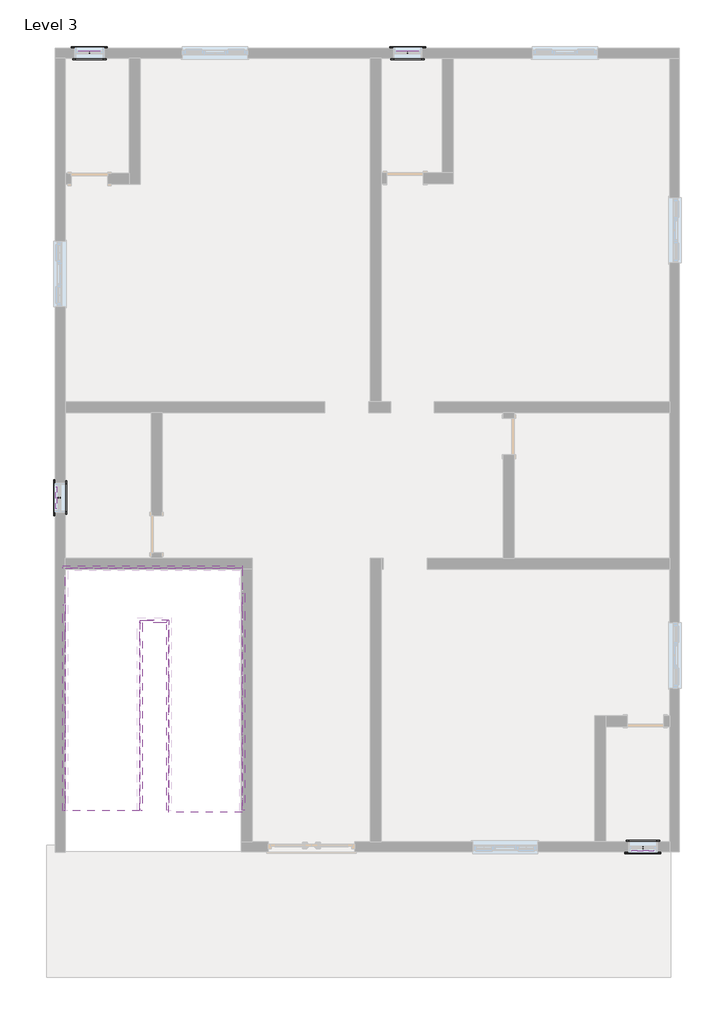
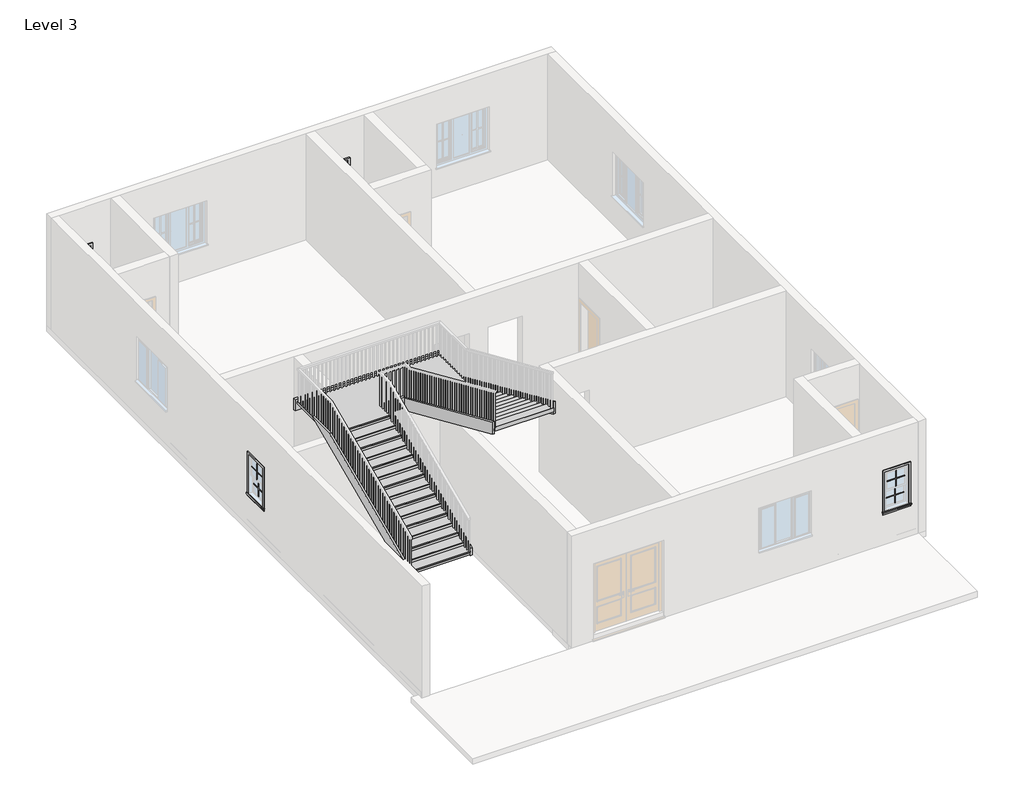
# One storey, part 6 of 6: 16 proxies, 12 members, 2 stair flights.
"""IFC4 building model written with IfcOpenShell, lengths in millimetres."""

from ifc_helpers import new_model, si_unit, frame, origin, place, context, project, spatial, polyline, outline, extrude, transform, mapped, element, save
from components import muntin_pattern_2x2_muntin_pattern_2x2_eba6c5fb, trim_window_exterior_flat_with_sill_278e6a94, trim_window_interior_flat_picture_frame_e9fd5f45, stair_flight_0f889a08

model = new_model("IFC4")

# Units and contexts
model_context = context("Model", 3, world=origin())
ifc_project = project(units=[si_unit("LENGTHUNIT", "METRE", prefix="MILLI")], contexts=[model_context])

# Site, building, storey
site = spatial("IfcSite", under=ifc_project)
building = spatial("IfcBuilding", under=site)
storey = spatial("IfcBuildingStorey", under=building, Name="Level 3", Elevation=6096.0)

# Proxies
placement = place(None, origin())
muntin_pattern_2x2_muntin_pattern_2x2_shape = muntin_pattern_2x2_muntin_pattern_2x2_eba6c5fb(model_context)
element("IfcBuildingElementProxy", 1, Name="Muntin Pattern_2x2 : Muntin Pattern_2x2", ObjectType="Muntin Pattern_2x2 : Muntin Pattern_2x2", at=placement, inside=storey, context=model_context, shape_type="MappedRepresentation", body=[
    mapped(muntin_pattern_2x2_muntin_pattern_2x2_shape, transform((-7722.7165084, -455.2217109, 7566.025), x_axis=(0.0, 1.0, 0.0), y_axis=(-1.0, 0.0, 0.0), z_axis=(0.0, 0.0, 1.0))),
])
element("IfcBuildingElementProxy", 2, Name="Muntin Pattern_2x2 : Muntin Pattern_2x2", ObjectType="Muntin Pattern_2x2 : Muntin Pattern_2x2", at=placement, inside=storey, context=model_context, shape_type="MappedRepresentation", body=[
    mapped(muntin_pattern_2x2_muntin_pattern_2x2_shape, transform((-7678.2665084, -455.2217109, 7086.6), x_axis=(0.0, 1.0, 0.0), y_axis=(-1.0, 0.0, 0.0), z_axis=(0.0, 0.0, 1.0))),
])
element("IfcBuildingElementProxy", 3, Name="Muntin Pattern_2x2 : Muntin Pattern_2x2", ObjectType="Muntin Pattern_2x2 : Muntin Pattern_2x2", at=placement, inside=storey, context=model_context, shape_type="MappedRepresentation", body=[
    mapped(muntin_pattern_2x2_muntin_pattern_2x2_shape, transform((-7046.4415084, 8872.5685985, 7566.025), x_axis=(1.0, 0.0, 0.0), y_axis=(0.0, 1.0, 0.0), z_axis=(0.0, 0.0, 1.0))),
])
element("IfcBuildingElementProxy", 4, Name="Muntin Pattern_2x2 : Muntin Pattern_2x2", ObjectType="Muntin Pattern_2x2 : Muntin Pattern_2x2", at=placement, inside=storey, context=model_context, shape_type="MappedRepresentation", body=[
    mapped(muntin_pattern_2x2_muntin_pattern_2x2_shape, transform((-7046.4415084, 8828.1185985, 7086.6), x_axis=(1.0, 0.0, 0.0), y_axis=(0.0, 1.0, 0.0), z_axis=(0.0, 0.0, 1.0))),
])
element("IfcBuildingElementProxy", 5, Name="Muntin Pattern_2x2 : Muntin Pattern_2x2", ObjectType="Muntin Pattern_2x2 : Muntin Pattern_2x2", at=placement, inside=storey, context=model_context, shape_type="MappedRepresentation", body=[
    mapped(muntin_pattern_2x2_muntin_pattern_2x2_shape, transform((-417.0415084, 8872.5685985, 7566.025), x_axis=(1.0, 0.0, 0.0), y_axis=(0.0, 1.0, 0.0), z_axis=(0.0, 0.0, 1.0))),
])
element("IfcBuildingElementProxy", 6, Name="Muntin Pattern_2x2 : Muntin Pattern_2x2", ObjectType="Muntin Pattern_2x2 : Muntin Pattern_2x2", at=placement, inside=storey, context=model_context, shape_type="MappedRepresentation", body=[
    mapped(muntin_pattern_2x2_muntin_pattern_2x2_shape, transform((-417.0415084, 8828.1185985, 7086.6), x_axis=(1.0, 0.0, 0.0), y_axis=(0.0, 1.0, 0.0), z_axis=(0.0, 0.0, 1.0))),
])
element("IfcBuildingElementProxy", 7, Name="Muntin Pattern_2x2 : Muntin Pattern_2x2", ObjectType="Muntin Pattern_2x2 : Muntin Pattern_2x2", at=placement, inside=storey, context=model_context, shape_type="MappedRepresentation", body=[
    mapped(muntin_pattern_2x2_muntin_pattern_2x2_shape, transform((4485.1584916, -7796.1814015, 7566.025), x_axis=(-1.0, 0.0, 0.0), y_axis=(0.0, -1.0, 0.0), z_axis=(0.0, 0.0, 1.0))),
])
element("IfcBuildingElementProxy", 8, Name="Muntin Pattern_2x2 : Muntin Pattern_2x2", ObjectType="Muntin Pattern_2x2 : Muntin Pattern_2x2", at=placement, inside=storey, context=model_context, shape_type="MappedRepresentation", body=[
    mapped(muntin_pattern_2x2_muntin_pattern_2x2_shape, transform((4485.1584916, -7751.7314015, 7086.6), x_axis=(-1.0, 0.0, 0.0), y_axis=(0.0, -1.0, 0.0), z_axis=(0.0, 0.0, 1.0))),
])
trim_window_exterior_flat_with_sill_shape = trim_window_exterior_flat_with_sill_278e6a94(model_context)
element("IfcBuildingElementProxy", 9, Name="Trim-Window-Exterior-Flat : with Sill", ObjectType="Trim-Window-Exterior-Flat : with Sill", at=placement, inside=storey, context=model_context, shape_type="MappedRepresentation", body=[
    mapped(trim_window_exterior_flat_with_sill_shape, transform((-7757.6415084, -455.2217109, 8077.2), x_axis=(0.0, -1.0, 0.0), y_axis=(0.0, 0.0, 1.0), z_axis=(-1.0, 0.0, 0.0))),
])
element("IfcBuildingElementProxy", 10, Name="Trim-Window-Exterior-Flat : with Sill", ObjectType="Trim-Window-Exterior-Flat : with Sill", at=placement, inside=storey, context=model_context, shape_type="MappedRepresentation", body=[
    mapped(trim_window_exterior_flat_with_sill_shape, transform((-7046.4415084, 8907.4935985, 8077.2), x_axis=(-1.0, 0.0, 0.0), y_axis=(0.0, 0.0, 1.0), z_axis=(0.0, 1.0, 0.0))),
])
element("IfcBuildingElementProxy", 11, Name="Trim-Window-Exterior-Flat : with Sill", ObjectType="Trim-Window-Exterior-Flat : with Sill", at=placement, inside=storey, context=model_context, shape_type="MappedRepresentation", body=[
    mapped(trim_window_exterior_flat_with_sill_shape, transform((-417.0415084, 8907.4935985, 8077.2), x_axis=(-1.0, 0.0, 0.0), y_axis=(0.0, 0.0, 1.0), z_axis=(0.0, 1.0, 0.0))),
])
element("IfcBuildingElementProxy", 12, Name="Trim-Window-Exterior-Flat : with Sill", ObjectType="Trim-Window-Exterior-Flat : with Sill", at=placement, inside=storey, context=model_context, shape_type="MappedRepresentation", body=[
    mapped(trim_window_exterior_flat_with_sill_shape, transform((4485.1584916, -7831.1064015, 8077.2), x_axis=(1.0, 0.0, 0.0), y_axis=(0.0, 0.0, 1.0), z_axis=(0.0, -1.0, 0.0))),
])
trim_window_interior_flat_picture_frame_shape = trim_window_interior_flat_picture_frame_e9fd5f45(model_context)
element("IfcBuildingElementProxy", 13, Name="Trim-Window-Interior-Flat : Picture Frame", ObjectType="Trim-Window-Interior-Flat : Picture Frame", at=placement, inside=storey, context=model_context, shape_type="MappedRepresentation", body=[
    mapped(trim_window_interior_flat_picture_frame_shape, transform((-7554.4415084, -455.2217109, 8077.2), x_axis=(0.0, 1.0, 0.0), y_axis=(0.0, 0.0, 1.0), z_axis=(1.0, 0.0, 0.0))),
])
element("IfcBuildingElementProxy", 14, Name="Trim-Window-Interior-Flat : Picture Frame", ObjectType="Trim-Window-Interior-Flat : Picture Frame", at=placement, inside=storey, context=model_context, shape_type="MappedRepresentation", body=[
    mapped(trim_window_interior_flat_picture_frame_shape, transform((-7046.4415084, 8704.2935985, 8077.2), x_axis=(1.0, 0.0, 0.0), y_axis=(0.0, 0.0, 1.0), z_axis=(0.0, -1.0, 0.0))),
])
element("IfcBuildingElementProxy", 15, Name="Trim-Window-Interior-Flat : Picture Frame", ObjectType="Trim-Window-Interior-Flat : Picture Frame", at=placement, inside=storey, context=model_context, shape_type="MappedRepresentation", body=[
    mapped(trim_window_interior_flat_picture_frame_shape, transform((-417.0415084, 8704.2935985, 8077.2), x_axis=(1.0, 0.0, 0.0), y_axis=(0.0, 0.0, 1.0), z_axis=(0.0, -1.0, 0.0))),
])
element("IfcBuildingElementProxy", 16, Name="Trim-Window-Interior-Flat : Picture Frame", ObjectType="Trim-Window-Interior-Flat : Picture Frame", at=placement, inside=storey, context=model_context, shape_type="MappedRepresentation", body=[
    mapped(trim_window_interior_flat_picture_frame_shape, transform((4485.1584916, -7627.9064015, 8077.2), x_axis=(-1.0, 0.0, 0.0), y_axis=(0.0, 0.0, 1.0), z_axis=(0.0, 1.0, 0.0))),
])

# Members
element("IfcMember", 17, ObjectType="Stringer - 2\" Width", at=placement, inside=storey, context=model_context, shape_type="SweptSolid", body=[
    extrude(outline(polyline([(-6973.0610642, 8839.2), (-6973.0610642, 9038.0550815), (-3441.822613, 10591.8), (-2685.0041973, 10591.8), (-6668.1860155, 8839.2), (-6973.0610642, 8839.2)])), frame((-7605.2415084, 0.0, 0.0), z_axis=(1.0, 0.0, 0.0), x_axis=(0.0, 1.0, 0.0)), (0.0, 0.0, 1.0), 50.8),
])
element("IfcMember", 18, ObjectType="Stringer - 2\" Width", at=placement, inside=storey, context=model_context, shape_type="SweptSolid", body=[
    extrude(outline(polyline([(-7605.2415084, -1928.4217109), (-7605.2415084, -1877.6217109), (-3866.3290366, -1877.6217109), (-3866.3290366, -1928.4217109), (-7605.2415084, -1928.4217109)])), frame((0.0, 0.0, 10287.0), z_axis=(0.0, 0.0, 1.0), x_axis=(1.0, 0.0, 0.0)), (0.0, 0.0, 1.0), 304.8),
])
element("IfcMember", 19, ObjectType="Stringer - 2\" Width", at=placement, inside=storey, context=model_context, shape_type="SweptSolid", body=[
    extrude(outline(polyline([(-3202.3906584, 10287.0), (-6973.0610642, 11946.0949786), (-6973.0610642, 12279.0950815), (-2445.5722427, 10287.0), (-3202.3906584, 10287.0)])), frame((-3866.3290366, 0.0, 0.0), z_axis=(1.0, 0.0, 0.0), x_axis=(0.0, 1.0, 0.0)), (0.0, 0.0, 1.0), 50.8),
])
element("IfcMember", 20, ObjectType="Stringer - 2\" Width", at=placement, inside=storey, context=model_context, shape_type="SweptSolid", body=[
    extrude(outline(polyline([(-6973.0610642, 8839.2), (-6973.0610642, 9038.0550815), (-3441.822613, 10591.8), (-3061.4610642, 10591.8), (-3061.4610642, 10426.1589786), (-6668.1860155, 8839.2), (-6973.0610642, 8839.2)])), frame((-5999.9290366, 0.0, 0.0), z_axis=(1.0, 0.0, 0.0), x_axis=(0.0, 1.0, 0.0)), (0.0, 0.0, 1.0), 50.8),
])
element("IfcMember", 21, ObjectType="Stringer - 2\" Width", at=placement, inside=storey, context=model_context, shape_type="SweptSolid", body=[
    extrude(outline(polyline([(-5999.9290366, -3061.4610642), (-5999.9290366, -3010.6610642), (-5441.1290366, -3010.6610642), (-5441.1290366, -3061.4610642), (-5999.9290366, -3061.4610642)])), frame((0.0, 0.0, 10287.0), z_axis=(0.0, 0.0, 1.0), x_axis=(1.0, 0.0, 0.0)), (0.0, 0.0, 1.0), 304.8),
])
element("IfcMember", 22, ObjectType="Stringer - 2\" Width", at=placement, inside=storey, context=model_context, shape_type="SweptSolid", body=[
    extrude(outline(polyline([(-3010.6610642, 10535.6390815), (-3010.6610642, 10287.0), (-3202.3906584, 10287.0), (-6973.0610642, 11946.0949786), (-6973.0610642, 12279.0950815), (-3010.6610642, 10535.6390815)])), frame((-5441.1290366, 0.0, 0.0), z_axis=(1.0, 0.0, 0.0), x_axis=(0.0, 1.0, 0.0)), (0.0, 0.0, 1.0), 50.8),
])
element("IfcMember", 23, ObjectType="Stringer - 2\" Width", at=placement, inside=storey, context=model_context, shape_type="SweptSolid", body=[
    extrude(outline(polyline([(-6973.0610642, 8839.2), (-6973.0610642, 9038.0550815), (-3441.822613, 10591.8), (-2685.0041973, 10591.8), (-6668.1860155, 8839.2), (-6973.0610642, 8839.2)])), frame((-7605.2415084, 0.0, 0.0), z_axis=(1.0, 0.0, 0.0), x_axis=(0.0, 1.0, 0.0)), (0.0, 0.0, 1.0), 50.8),
])
element("IfcMember", 24, ObjectType="Stringer - 2\" Width", at=placement, inside=storey, context=model_context, shape_type="SweptSolid", body=[
    extrude(outline(polyline([(-7605.2415084, -1928.4217109), (-7605.2415084, -1877.6217109), (-3866.3290366, -1877.6217109), (-3866.3290366, -1928.4217109), (-7605.2415084, -1928.4217109)])), frame((0.0, 0.0, 10287.0), z_axis=(0.0, 0.0, 1.0), x_axis=(1.0, 0.0, 0.0)), (0.0, 0.0, 1.0), 304.8),
])
element("IfcMember", 25, ObjectType="Stringer - 2\" Width", at=placement, inside=storey, context=model_context, shape_type="SweptSolid", body=[
    extrude(outline(polyline([(-3202.3906584, 10287.0), (-6973.0610642, 11946.0949786), (-6973.0610642, 12279.0950815), (-2445.5722427, 10287.0), (-3202.3906584, 10287.0)])), frame((-3866.3290366, 0.0, 0.0), z_axis=(1.0, 0.0, 0.0), x_axis=(0.0, 1.0, 0.0)), (0.0, 0.0, 1.0), 50.8),
])
element("IfcMember", 26, ObjectType="Stringer - 2\" Width", at=placement, inside=storey, context=model_context, shape_type="SweptSolid", body=[
    extrude(outline(polyline([(-6973.0610642, 8839.2), (-6973.0610642, 9038.0550815), (-3441.822613, 10591.8), (-3061.4610642, 10591.8), (-3061.4610642, 10426.1589786), (-6668.1860155, 8839.2), (-6973.0610642, 8839.2)])), frame((-5999.9290366, 0.0, 0.0), z_axis=(1.0, 0.0, 0.0), x_axis=(0.0, 1.0, 0.0)), (0.0, 0.0, 1.0), 50.8),
])
element("IfcMember", 27, ObjectType="Stringer - 2\" Width", at=placement, inside=storey, context=model_context, shape_type="SweptSolid", body=[
    extrude(outline(polyline([(-5999.9290366, -3061.4610642), (-5999.9290366, -3010.6610642), (-5441.1290366, -3010.6610642), (-5441.1290366, -3061.4610642), (-5999.9290366, -3061.4610642)])), frame((0.0, 0.0, 10287.0), z_axis=(0.0, 0.0, 1.0), x_axis=(1.0, 0.0, 0.0)), (0.0, 0.0, 1.0), 304.8),
])
element("IfcMember", 28, ObjectType="Stringer - 2\" Width", at=placement, inside=storey, context=model_context, shape_type="SweptSolid", body=[
    extrude(outline(polyline([(-3010.6610642, 10535.6390815), (-3010.6610642, 10287.0), (-3202.3906584, 10287.0), (-6973.0610642, 11946.0949786), (-6973.0610642, 12279.0950815), (-3010.6610642, 10535.6390815)])), frame((-5441.1290366, 0.0, 0.0), z_axis=(1.0, 0.0, 0.0), x_axis=(0.0, 1.0, 0.0)), (0.0, 0.0, 1.0), 50.8),
])

# Stair flights
stair_flight_shape = stair_flight_0f889a08(model_context)
element("IfcStairFlight", 29, ObjectType="2\" Tread 1\" Nosing 1/4\" Riser", at=placement, inside=storey, context=model_context, shape_type="MappedRepresentation", body=[
    mapped(stair_flight_shape, transform((0.0, 0.0, 0.0), x_axis=(1.0, 0.0, 0.0), y_axis=(0.0, 1.0, 0.0), z_axis=(0.0, 0.0, 1.0))),
])
element("IfcStairFlight", 30, ObjectType="2\" Tread 1\" Nosing 1/4\" Riser", at=placement, inside=storey, context=model_context, shape_type="MappedRepresentation", body=[
    mapped(stair_flight_shape, transform((0.0, 0.0, 0.0), x_axis=(1.0, 0.0, 0.0), y_axis=(0.0, 1.0, 0.0), z_axis=(0.0, 0.0, 1.0))),
])

save(model, "model.ifc")

# Revit data of these elements
# Type "Muntin Pattern_2x2 : Muntin Pattern_2x2"
#   Width [instance default] = 4' - 0"
#   Thickness = 0' - 0 1/2"
#   Height [instance default] = 4' - 0"
#   Distance = 0' - 0 3/4"
#   Interior Material [instance default] = none
#   Exterior Material [instance default] = none
#   Default Elevation = 0
# Type "Trim-Window-Exterior-Flat : with Sill"
#   Trim Width = 0' - 2 1/4"
#   Trim Thickness_Picture Frame = 0' - 1 1/4"
#   Trim Thickness_with Sill = 0' - 0 3/4"
#   Sill Thickness = 0' - 1 1/4"
#   Opening Width [instance default] = 2' - 0"
#   Opening Height [instance default] = 3' - 0"
#   Default Elevation = 4' - 0"
#   Sill = yes
#   Picture Frame = no
#   Trim Material [instance default] = none
# Type "Trim-Window-Interior-Flat : Picture Frame"
#   Trim Thickness_Picture Frame = 0' - 1 1/4"
#   Trim Width = 0' - 2 1/4"
#   Trim Thickness_with Sill = 0' - 0 3/4"
#   Sill Thickness = 0' - 1 1/4"
#   Opening Width [instance default] = 2' - 0"
#   Opening Height [instance default] = 3' - 0"
#   Default Elevation = 4' - 0"
#   Sill = no
#   Picture Frame = yes
#   Trim Material [instance default] = none
# Elements 1, 2, 3, 4, 5, 6, 7, 8 (IfcBuildingElementProxy, "Muntin Pattern_2x2 : Muntin Pattern_2x2")
#   Width = 1' - 6"
#   Height = 1' - 5 1/8"
#   Interior Material = Wood - Stained
#   Exterior Material = Clad - White
#   Phase Created = New Construction
#   Materials on its faces: "Clad - White", "Wood - Stained"
# Elements 9, 10, 11, 12 (IfcBuildingElementProxy, "Trim-Window-Exterior-Flat : with Sill")
#   Opening Width = 2' - 0"
#   Opening Height = 3' - 6"
#   Trim Material = Clad - White
#   Phase Created = New Construction
#   Materials on its faces: "Clad - White"
# Elements 13, 14, 15, 16 (IfcBuildingElementProxy, "Trim-Window-Interior-Flat : Picture Frame")
#   Opening Width = 2' - 0"
#   Opening Height = 3' - 6"
#   Trim Material = Wood - Stained
#   Phase Created = New Construction
#   Materials on its faces: "Wood - Stained"
# Elements 17, 18, 19, 20, 21, 22, 23, 24, 25, 26, 27, 28 (IfcMember, "Stringer - 2\" Width")
#   Phase Created = New Construction
# Elements 29, 30 (IfcStairFlight, "2\" Tread 1\" Nosing 1/4\" Riser")
#   Phase Created = New Construction
# Materials
#   "Clad - White": class "Wood", colour RGB 242 242 238, transparency 0, Cost = 0
#   "Wood - Stained": class "Wood", colour RGB 224 178 126, transparency 0, Cost = 0
